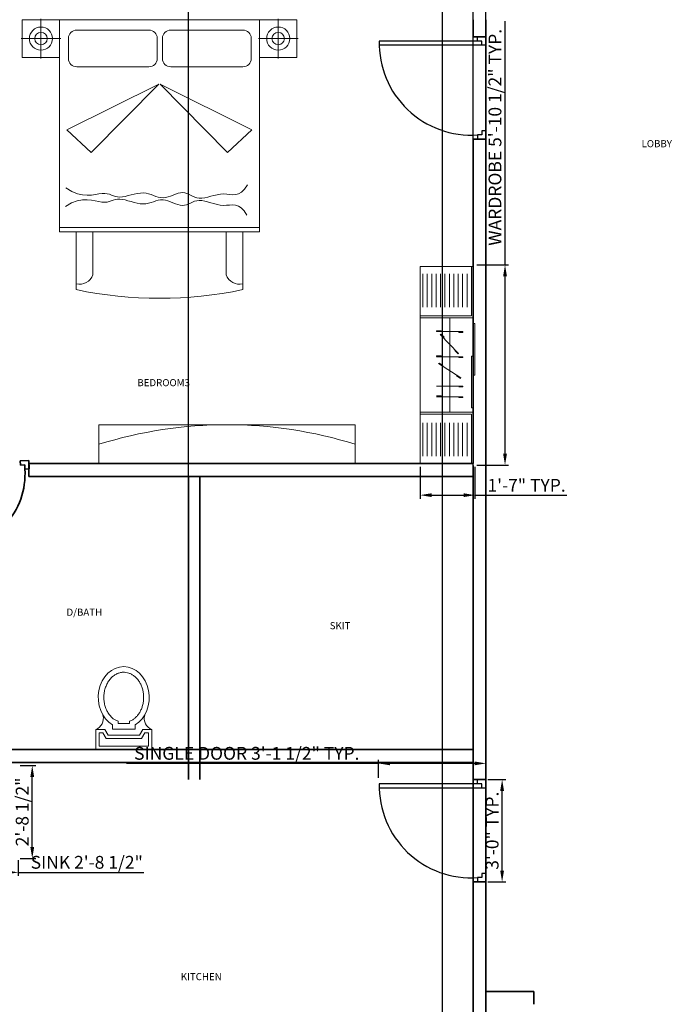
# Model space of a CAD drawing. Units: inches. Extents: x 1239 to 2276906, y 2273 to 321338.
# Tile 16 of 23: x 1392 to 1620, y 3026 to 3372. Entities that reach past the tile are written whole.
import ezdxf

# ---------------------------------------------------------------- set-up
doc = ezdxf.new("R2010")
doc.units = ezdxf.units.IN
for name, color, linetype, lineweight in [('A-ANNO-DIMS', 2, 'Continuous', 18), ('A-AREA-IDEN', 7, 'Continuous', 18), ('A-FLOR-CASE', 8, 'Continuous', 18), ('A-FLOR-FIXT', 9, 'Continuous', 18), ('A-FURN', 8, 'Continuous', 13), ('DOOR', 1, 'Continuous', 25), ('wall', 7, 'Continuous', 35)]:
    doc.layers.add(name, color=color, linetype=linetype, lineweight=lineweight)
doc.styles.get("Standard").update_dxf_attribs({"font": 'arial.ttf'})
doc.dimstyles.new('ISO-25', dxfattribs={"dimtxt": 4.5, "dimasz": 4, "dimexe": 1.25, "dimexo": 0.625, "dimtad": 1, "dimdec": 1, "dimlunit": 3, "dimtxsty": 'Standard', "dimcen": 2.5, "dimadec": 0, "dimazin": 0, "dimtfac": 1, "dimtdec": 1, "dimtmove": 0, "dimatfit": 3, "dimfxl": 1, "dimarcsym": 0})

# ---------------------------------------------------------------- blocks, each defined once
blk = doc.blocks.new('new block')
for p, q in [((1.5, 1.5), (1.5, 30)), ((3, 0), (3, 30)), ((0, 3), (0, 0)), ((1.5, 3), (0, 3)), ((0, 0), (3, 0)), ((1.5, 1.5), (1.5, 3)), ((3, 1.5), (1.5, 1.5)), ((3, 0), (3, 1.5)), ((27, 0), (27, 1.5)), ((27, 1.5), (28.5, 1.5)), ((30, 0), (27, 0)), ((28.5, 1.5), (28.5, 3)), ((28.5, 3), (30, 3)), ((30, 3), (30, 0))]:
    blk.add_line(p, q)
blk.add_arc((2.25, 3.75), 26.26, 358.3634, 91.6366)
blk = doc.blocks.new('2.6door')
at = {"layer": 'wall'}
blk.add_blockref('new block', (0, 0), dxfattribs=at)
blk = doc.blocks.new('A$C4F543DC7')
for p, q in [((0.013, 3.35, -0.169), (3.313, 3.35, -0.169)), ((0.463, 3.35, -0.169), (0.013, 3.35, -0.169)), ((0.013, 2.896, -0.169), (0.013, 3.35, -0.169)), ((0.013, 3.35, -0.169), (0.013, 2.896, -0.169)), ((0.238, 3.123, -0.439), (0.238, 3.361, -0.439)), ((0.463, 3.35, -0.169), (0.463, 0.8, -0.169)), ((2.863, 3.35, -0.169), (0.463, 3.35, -0.169)), ((0.463, 2.896, -0.169), (0.463, 3.35, -0.169)), ((2.863, 0.8, -0.169), (2.863, 3.35, -0.169)), ((2.863, 3.35, -0.169), (3.313, 3.35, -0.169)), ((2.863, 2.896, -0.169), (2.863, 3.35, -0.169)), ((3.089, 3.123, -0.439), (3.089, 3.361, -0.439)), ((3.313, 3.35, -0.169), (3.313, 2.896, -0.169)), ((3.313, 3.35, -0.169), (3.313, 2.896, -0.169)), ((1.535, 3.226, -0.169), (0.668, 3.226, -0.169)), ((2.664, 3.226, -0.169), (1.797, 3.226, -0.169)), ((0.238, 3.123, -0.439), (0, 3.123, -0.439)), ((0.238, 3.123, -0.439), (0.476, 3.123, -0.439)), ((0.238, 3.123, -0.439), (0.238, 2.885, -0.439)), ((0.568, 3.126, -0.169), (0.568, 2.884, -0.169)), ((1.635, 2.884, -0.169), (1.635, 3.126, -0.169)), ((1.697, 3.126, -0.169), (1.697, 2.884, -0.169)), ((2.764, 2.884, -0.169), (2.764, 3.126, -0.169)), ((3.089, 3.123, -0.439), (2.851, 3.123, -0.439)), ((3.089, 3.123, -0.439), (3.089, 2.885, -0.439)), ((3.089, 3.123, -0.439), (3.327, 3.123, -0.439)), ((0.463, 2.896, -0.169), (0.013, 2.896, -0.169)), ((0.013, 2.896, -0.169), (0.463, 2.896, -0.169)), ((0.463, 0.8, -0.169), (0.463, 2.896, -0.169)), ((2.863, 2.896, -0.169), (2.863, 0.8, -0.169)), ((3.313, 2.896, -0.169), (2.863, 2.896, -0.169)), ((3.313, 2.896, -0.169), (2.863, 2.896, -0.169)), ((0.668, 2.784, -0.169), (1.535, 2.784, -0.169)), ((1.797, 2.784, -0.169), (2.664, 2.784, -0.169)), ((1.653, 2.573, -0.169), (0.55, 2.025, -0.169)), ((0.841, 1.752, -0.169), (1.653, 2.573, -0.169)), ((2.481, 1.752, -0.169), (1.669, 2.573, -0.169)), ((1.669, 2.573, -0.169), (2.772, 2.025, -0.169)), ((0.55, 2.025, -0.169), (0.841, 1.752, -0.169)), ((2.772, 2.025, -0.169), (2.481, 1.752, -0.169)), ((0.537, 1.327, -0.169), (0.609, 1.284, -0.169)), ((2.648, 1.277, -0.169), (2.683, 1.312, -0.169)), ((2.683, 1.312, -0.169), (2.718, 1.364, -0.169)), ((0.609, 1.284, -0.169), (0.676, 1.257, -0.169)), ((0.676, 1.257, -0.169), (0.737, 1.243, -0.169)), ((0.736, 1.183, -0.169), (0.793, 1.185, -0.169)), ((0.737, 1.243, -0.169), (0.794, 1.239, -0.169)), ((0.793, 1.185, -0.169), (0.845, 1.18, -0.169)), ((0.794, 1.239, -0.169), (0.846, 1.242, -0.169)), ((0.846, 1.242, -0.169), (0.893, 1.249, -0.169)), ((0.893, 1.249, -0.169), (0.935, 1.256, -0.169)), ((0.935, 1.256, -0.169), (0.972, 1.261, -0.169)), ((0.972, 1.261, -0.169), (1.004, 1.262, -0.169)), ((1.004, 1.262, -0.169), (1.033, 1.258, -0.169)), ((1.033, 1.258, -0.169), (1.06, 1.251, -0.169)), ((1.06, 1.251, -0.169), (1.084, 1.242, -0.169)), ((1.084, 1.242, -0.169), (1.108, 1.234, -0.169)), ((1.107, 1.18, -0.169), (1.132, 1.187, -0.169)), ((1.108, 1.234, -0.169), (1.132, 1.226, -0.169)), ((1.132, 1.226, -0.169), (1.158, 1.22, -0.169)), ((1.132, 1.187, -0.169), (1.157, 1.192, -0.169)), ((1.157, 1.192, -0.169), (1.185, 1.193, -0.169)), ((1.158, 1.22, -0.169), (1.185, 1.218, -0.169)), ((1.185, 1.218, -0.169), (1.216, 1.22, -0.169)), ((1.185, 1.193, -0.169), (1.216, 1.19, -0.169)), ((1.216, 1.22, -0.169), (1.25, 1.226, -0.169)), ((1.216, 1.19, -0.169), (1.249, 1.183, -0.169)), ((1.25, 1.226, -0.169), (1.285, 1.235, -0.169)), ((1.285, 1.235, -0.169), (1.322, 1.244, -0.169)), ((1.322, 1.244, -0.169), (1.359, 1.253, -0.169)), ((1.359, 1.253, -0.169), (1.396, 1.261, -0.169)), ((1.396, 1.261, -0.169), (1.433, 1.266, -0.169)), ((1.433, 1.266, -0.169), (1.468, 1.268, -0.169)), ((1.468, 1.268, -0.169), (1.501, 1.264, -0.169)), ((1.501, 1.264, -0.169), (1.532, 1.257, -0.169)), ((1.532, 1.257, -0.169), (1.562, 1.247, -0.169)), ((1.562, 1.247, -0.169), (1.591, 1.237, -0.169)), ((1.591, 1.237, -0.169), (1.62, 1.226, -0.169)), ((1.62, 1.226, -0.169), (1.648, 1.217, -0.169)), ((1.648, 1.217, -0.169), (1.676, 1.211, -0.169)), ((1.648, 1.18, -0.169), (1.676, 1.185, -0.169)), ((1.676, 1.211, -0.169), (1.705, 1.209, -0.169)), ((1.676, 1.185, -0.169), (1.705, 1.186, -0.169)), ((1.705, 1.209, -0.169), (1.735, 1.212, -0.169)), ((1.705, 1.186, -0.169), (1.734, 1.182, -0.169)), ((1.735, 1.212, -0.169), (1.765, 1.22, -0.169)), ((1.765, 1.22, -0.169), (1.795, 1.23, -0.169)), ((1.795, 1.23, -0.169), (1.826, 1.242, -0.169)), ((1.826, 1.242, -0.169), (1.856, 1.253, -0.169)), ((1.856, 1.253, -0.169), (1.885, 1.263, -0.169)), ((1.885, 1.263, -0.169), (1.913, 1.27, -0.169)), ((1.913, 1.27, -0.169), (1.94, 1.272, -0.169)), ((1.94, 1.272, -0.169), (1.965, 1.269, -0.169)), ((1.965, 1.269, -0.169), (1.989, 1.262, -0.169)), ((1.989, 1.262, -0.169), (2.012, 1.251, -0.169)), ((2.012, 1.251, -0.169), (2.036, 1.239, -0.169)), ((2.036, 1.239, -0.169), (2.06, 1.227, -0.169)), ((2.06, 1.227, -0.169), (2.085, 1.216, -0.169)), ((2.085, 1.216, -0.169), (2.112, 1.208, -0.169)), ((2.112, 1.208, -0.169), (2.141, 1.204, -0.169)), ((2.141, 1.204, -0.169), (2.172, 1.205, -0.169)), ((2.172, 1.205, -0.169), (2.206, 1.21, -0.169)), ((2.206, 1.21, -0.169), (2.242, 1.218, -0.169)), ((2.242, 1.218, -0.169), (2.279, 1.228, -0.169)), ((2.279, 1.228, -0.169), (2.317, 1.238, -0.169)), ((2.317, 1.238, -0.169), (2.356, 1.246, -0.169)), ((2.356, 1.246, -0.169), (2.394, 1.253, -0.169)), ((2.394, 1.253, -0.169), (2.433, 1.255, -0.169)), ((2.433, 1.255, -0.169), (2.47, 1.253, -0.169)), ((2.47, 1.253, -0.169), (2.506, 1.249, -0.169)), ((2.506, 1.249, -0.169), (2.542, 1.246, -0.169)), ((2.542, 1.246, -0.169), (2.578, 1.248, -0.169)), ((2.578, 1.248, -0.169), (2.613, 1.257, -0.169)), ((2.613, 1.257, -0.169), (2.648, 1.277, -0.169)), ((0.533, 1.105, -0.169), (0.607, 1.146, -0.169)), ((0.607, 1.146, -0.169), (0.674, 1.171, -0.169)), ((0.674, 1.171, -0.169), (0.736, 1.183, -0.169)), ((0.845, 1.18, -0.169), (0.891, 1.172, -0.169)), ((0.891, 1.172, -0.169), (0.933, 1.163, -0.169)), ((0.933, 1.163, -0.169), (0.97, 1.156, -0.169)), ((0.97, 1.156, -0.169), (1.003, 1.155, -0.169)), ((1.003, 1.155, -0.169), (1.032, 1.158, -0.169)), ((1.032, 1.158, -0.169), (1.058, 1.164, -0.169)), ((1.058, 1.164, -0.169), (1.083, 1.172, -0.169)), ((1.083, 1.172, -0.169), (1.107, 1.18, -0.169)), ((1.249, 1.183, -0.169), (1.284, 1.173, -0.169)), ((1.284, 1.173, -0.169), (1.321, 1.163, -0.169)), ((1.321, 1.163, -0.169), (1.358, 1.152, -0.169)), ((1.358, 1.152, -0.169), (1.394, 1.143, -0.169)), ((1.394, 1.143, -0.169), (1.431, 1.137, -0.169)), ((1.431, 1.137, -0.169), (1.466, 1.135, -0.169)), ((1.466, 1.135, -0.169), (1.499, 1.137, -0.169)), ((1.499, 1.137, -0.169), (1.531, 1.143, -0.169)), ((1.531, 1.143, -0.169), (1.561, 1.152, -0.169)), ((1.561, 1.152, -0.169), (1.59, 1.162, -0.169)), ((1.59, 1.162, -0.169), (1.619, 1.172, -0.169)), ((1.619, 1.172, -0.169), (1.648, 1.18, -0.169)), ((1.734, 1.182, -0.169), (1.764, 1.173, -0.169)), ((1.764, 1.173, -0.169), (1.794, 1.162, -0.169)), ((1.794, 1.162, -0.169), (1.824, 1.149, -0.169)), ((1.824, 1.149, -0.169), (1.854, 1.137, -0.169)), ((1.854, 1.137, -0.169), (1.883, 1.126, -0.169)), ((1.883, 1.126, -0.169), (1.911, 1.119, -0.169)), ((1.911, 1.119, -0.169), (1.937, 1.115, -0.169)), ((1.937, 1.115, -0.169), (1.963, 1.118, -0.169)), ((1.963, 1.118, -0.169), (1.987, 1.124, -0.169)), ((1.987, 1.124, -0.169), (2.011, 1.134, -0.169)), ((2.011, 1.134, -0.169), (2.034, 1.145, -0.169)), ((2.034, 1.145, -0.169), (2.059, 1.157, -0.169)), ((2.059, 1.157, -0.169), (2.084, 1.167, -0.169)), ((2.084, 1.167, -0.169), (2.111, 1.174, -0.169)), ((2.111, 1.174, -0.169), (2.14, 1.177, -0.169)), ((2.14, 1.177, -0.169), (2.172, 1.175, -0.169)), ((2.172, 1.175, -0.169), (2.206, 1.169, -0.169)), ((2.206, 1.169, -0.169), (2.241, 1.16, -0.169)), ((2.241, 1.16, -0.169), (2.278, 1.149, -0.169)), ((2.278, 1.149, -0.169), (2.316, 1.138, -0.169)), ((2.316, 1.138, -0.169), (2.354, 1.128, -0.169)), ((2.354, 1.128, -0.169), (2.392, 1.121, -0.169)), ((2.392, 1.121, -0.169), (2.43, 1.117, -0.169)), ((2.43, 1.117, -0.169), (2.468, 1.118, -0.169)), ((2.468, 1.118, -0.169), (2.504, 1.121, -0.169)), ((2.504, 1.121, -0.169), (2.54, 1.123, -0.169)), ((2.54, 1.123, -0.169), (2.576, 1.12, -0.169)), ((2.576, 1.12, -0.169), (2.611, 1.109, -0.169)), ((2.611, 1.109, -0.169), (2.645, 1.088, -0.169)), ((2.645, 1.088, -0.169), (2.679, 1.052, -0.169)), ((2.679, 1.052, -0.169), (2.712, 0.999, -0.169)), ((0.463, 0.85, -0.169), (2.863, 0.85, -0.169)), ((0.463, 0.8, -0.169), (2.863, 0.8, -0.169)), ((0.663, 0.8, -0.169), (0.463, 0.8, -0.169)), ((0.663, 0.8, -0.169), (2.663, 0.8, -0.169)), ((0.663, 0.104, -0.169), (0.663, 0.8, -0.169)), ((0.663, 0.104, -0.169), (0.663, 0.8, -0.169)), ((0.863, 0.281, -0.169), (0.863, 0.8, -0.169)), ((2.463, 0.8, -0.169), (2.463, 0.281, -0.169)), ((2.863, 0.8, -0.169), (2.663, 0.8, -0.169)), ((2.663, 0.8, -0.169), (2.663, 0.104, -0.169)), ((2.663, 0.8, -0.169), (2.663, 0.104, -0.169))]:
    blk.add_line(p, q)
for centre, radius in [((0.238, 3.123, -0.439), 0.139), ((0.238, 3.123, -0.439), 0.075), ((3.089, 3.123, -0.439), 0.139), ((3.089, 3.123, -0.439), 0.075)]:
    blk.add_circle(centre, radius)
for centre, radius, start, end in [((0.668, 3.126, -0.169), 0.1, 90, 180), ((1.535, 3.126, -0.169), 0.1, 0, 90), ((1.797, 3.126, -0.169), 0.1, 90, 180), ((2.664, 3.126, -0.169), 0.1, 0, 90), ((0.668, 2.884, -0.169), 0.1, 180, 270), ((1.535, 2.884, -0.169), 0.1, 270, 0), ((1.797, 2.884, -0.169), 0.1, 180, 270), ((2.664, 2.884, -0.169), 0.1, 270, 0), ((0.699, 0.347, -0.169), 0.177, 258.2616, 338.032), ((2.627, 0.347, -0.169), 0.177, 201.968, 281.7384), ((1.663, 4.86, -0.169), 4.86, 258.1252, 281.8748), ((1.663, 4.86, -0.169), 4.86, 258.1252, 281.8748)]:
    blk.add_arc(centre, radius, start, end)
blk = doc.blocks.new('A$C34930FF8')
at = {"ltscale": 0.05}
for p, q in [((0, 2252), (0, 17)), ((600, 2252), (0, 2252)), ((185, 1513), (185, 1521)), ((227, 1479), (233, 1485)), ((238, 1513), (238, 1521)), ((437, 1513), (437, 1504)), ((482, 1513), (482, 1504)), ((264, 1442), (270, 1448)), ((185, 1229), (185, 1238)), ((238, 1229), (238, 1238)), ((398, 1304), (392, 1298)), ((435, 1266), (429, 1260)), ((437, 1228), (437, 1220)), ((482, 1228), (482, 1220)), ((209, 1150), (214, 1157)), ((253, 1122), (258, 1129)), ((415, 1018), (411, 1010)), ((459, 989), (455, 982)), ((482, 895), (482, 886)), ((238, 775), (238, 784)), ((437, 775), (437, 767)), ((482, 775), (482, 767)), ((600, 17), (0, 17))]:
    blk.add_line(p, q, dxfattribs=at)
for p, q in [((580, 1691), (580, 2252)), ((600, 1669), (600, 2269)), ((30, 1791), (30, 2169)), ((80, 1791), (80, 2169)), ((130, 1791), (130, 2169)), ((180, 1791), (180, 2169)), ((230, 1791), (230, 2169)), ((280, 1791), (280, 2169)), ((330, 1791), (330, 2169)), ((380, 1791), (380, 2169)), ((430, 1791), (430, 2169)), ((480, 1791), (480, 2169)), ((530, 1791), (530, 2169)), ((580, 1691), (0, 1691)), ((600, 1669), (0, 1669)), ((335, 1666), (335, 603)), ((600, 1603), (620, 1603)), ((600, 1019), (600, 1603)), ((620, 1603), (620, 1019)), ((238, 1521), (185, 1521)), ((482, 1513), (185, 1513)), ((435, 1266), (227, 1479)), ((270, 1448), (233, 1485)), ((437, 1504), (482, 1504)), ((238, 1238), (185, 1238)), ((482, 1228), (185, 1228)), ((429, 1260), (392, 1298)), ((600, 1233), (580, 1233)), ((580, 1233), (580, 649)), ((600, 649), (600, 1233)), ((459, 989), (209, 1150)), ((258, 1129), (214, 1157)), ((437, 1220), (482, 1220)), ((455, 982), (411, 1010)), ((620, 1019), (600, 1019)), ((482, 895), (185, 895)), ((238, 784), (185, 784)), ((437, 886), (482, 886)), ((482, 775), (185, 775)), ((437, 767), (482, 767)), ((600, 600), (0, 600)), ((580, 578), (0, 578)), ((580, 649), (600, 649)), ((580, 578), (580, 17)), ((600, 600), (600, 0)), ((30, 478), (30, 100)), ((80, 478), (80, 100)), ((130, 478), (130, 100)), ((180, 478), (180, 100)), ((230, 478), (230, 100)), ((280, 478), (280, 100)), ((330, 478), (330, 100)), ((380, 478), (380, 100)), ((430, 478), (430, 100)), ((480, 478), (480, 100)), ((530, 478), (530, 100))]:
    blk.add_line(p, q)
blk = doc.blocks.new('A$C7C8779AE')
for p, q in [((0, 0.7405), (0, 0.5605)), ((0.5, 0.7405), (0, 0.7405)), ((0.47, 0.7105), (0.03, 0.7105)), ((0.03, 0.7105), (0.03, 0.5905)), ((0.47, 0.5905), (0.47, 0.7105)), ((0.5, 0.5605), (0.5, 0.7405)), ((0.093, 0.6405), (0.063, 0.5905)), ((0.093, 0.6405), (0.407, 0.6405)), ((0.437, 0.5905), (0.407, 0.6405)), ((0, 0.5605), (0.08, 0.5605)), ((0.03, 0.5905), (0.063, 0.5905)), ((0.11, 0.6105), (0.08, 0.5605)), ((0.11, 0.6105), (0.39, 0.6105)), ((0.1497, 0.557), (0.1497, 0.5203)), ((0.1497, 0.557), (0.3514, 0.557)), ((0.3514, 0.557), (0.3514, 0.5203)), ((0.42, 0.5605), (0.39, 0.6105)), ((0.42, 0.5605), (0.5, 0.5605)), ((0.437, 0.5905), (0.47, 0.5905)), ((0.1997, 0.507), (0.1997, 0.4879)), ((0.1997, 0.507), (0.3014, 0.507)), ((0.3014, 0.507), (0.3014, 0.4879))]:
    blk.add_line(p, q)
for centre, start, end in [((-0.0386, 0.4613), 344.64203, 68.73386), ((0.5386, 0.4613), 111.26614, 195.35797)]:
    blk.add_arc(centre, 0.1064, start, end)
blk.add_ellipse((0.2506, 0.2744), major_axis=(0, 0.2744), ratio=0.828948, start_param=0.459479, end_param=5.823706)
blk.add_open_spline([(0.1997, 0.4879), (0.1697, 0.474), (0.1642, 0.4702), (0.1512, 0.4602), (0.1438, 0.4535), (0.1298, 0.4388), (0.1233, 0.4306), (0.1111, 0.4131), (0.1055, 0.4037), (0.0956, 0.3838), (0.0912, 0.3733), (0.0838, 0.3516), (0.0808, 0.3403), (0.0762, 0.3172), (0.0746, 0.3055), (0.073, 0.2817), (0.0729, 0.2698), (0.0743, 0.246), (0.0758, 0.2342), (0.0801, 0.2111), (0.0831, 0.1998), (0.0903, 0.1779), (0.0945, 0.1673), (0.1043, 0.1473), (0.1098, 0.1378), (0.1218, 0.12), (0.1283, 0.1118), (0.1421, 0.0968), (0.1494, 0.09), (0.1646, 0.078), (0.1725, 0.0728), (0.1887, 0.064), (0.1969, 0.0603), (0.2137, 0.0547), (0.2222, 0.0527), (0.2392, 0.0502), (0.2478, 0.0498), (0.2664, 0.0505), (0.2764, 0.052), (0.2963, 0.0573), (0.3061, 0.061), (0.3253, 0.0707), (0.3346, 0.0766), (0.3525, 0.0906), (0.3611, 0.0987), (0.3771, 0.1169), (0.3845, 0.127), (0.3978, 0.1488), (0.4037, 0.1605), (0.4137, 0.1853), (0.4178, 0.1983), (0.424, 0.2251), (0.4261, 0.2389), (0.4282, 0.2668), (0.4283, 0.2809), (0.4262, 0.3088), (0.4241, 0.3226), (0.418, 0.3495), (0.414, 0.3625), (0.404, 0.3873), (0.3982, 0.3991), (0.385, 0.421), (0.3776, 0.4311), (0.3617, 0.4494), (0.3531, 0.4575), (0.3382, 0.4693), (0.3321, 0.4736), (0.3014, 0.4879)], degree=3, knots=[0.459479, 0.459479, 0.459479, 0.459479, 0.567422, 0.567422, 0.720865, 0.720865, 0.874307, 0.874307, 1.02775, 1.02775, 1.181192, 1.181192, 1.334635, 1.334635, 1.488077, 1.488077, 1.64152, 1.64152, 1.794963, 1.794963, 1.948405, 1.948405, 2.101848, 2.101848, 2.25529, 2.25529, 2.408733, 2.408733, 2.562175, 2.562175, 2.715618, 2.715618, 2.86906, 2.86906, 3.022503, 3.022503, 3.175946, 3.175946, 3.356457, 3.356457, 3.536968, 3.536968, 3.717479, 3.717479, 3.89799, 3.89799, 4.078501, 4.078501, 4.259012, 4.259012, 4.439523, 4.439523, 4.620035, 4.620035, 4.800546, 4.800546, 4.981057, 4.981057, 5.161568, 5.161568, 5.342079, 5.342079, 5.52259, 5.52259, 5.703101, 5.703101, 5.823706, 5.823706, 5.823706, 5.823706])
blk = doc.blocks.new('DOOR-SINGLE-36')
for p, q in [((33, 1.5), (33, 37.5)), ((34.5, 1.5), (34.5, 37.5)), ((0, 3), (0, 0)), ((1.5, 3), (0, 3)), ((0, 0), (3, 0)), ((1.5, 1.5), (1.5, 3)), ((3, 1.5), (1.5, 1.5)), ((3, 0), (3, 1.5)), ((33, 0), (33, 1.5)), ((33, 1.5), (34.5, 1.5)), ((36, 0), (33, 0)), ((34.5, 1.5), (34.5, 3)), ((34.5, 3), (36, 3)), ((36, 3), (36, 0))]:
    blk.add_line(p, q)
blk.add_arc((33.75, 5.18), 32.32, 88.6705, 183.8756)
blk = doc.blocks.new('*D48')
at = {"layer": 'A-ANNO-DIMS', "color": 0, "lineweight": -2, "transparency": 16777216}
for p, q in [((1518.17, 3111.05), (1429.62, 3111.05)), ((1518.17, 3106.02), (1518.17, 3112.3)), ((1551.88, 3111.05), (1522.17, 3111.05)), ((1555.88, 3106.02), (1555.88, 3112.3))]:
    blk.add_line(p, q, dxfattribs=at)
at = {"layer": 'A-ANNO-DIMS', "color": 0, "transparency": 16777216}
for points in [[(1522.17, 3111.72), (1522.17, 3110.39), (1518.17, 3111.05)], [(1551.88, 3111.72), (1551.88, 3110.39), (1555.88, 3111.05)]]:
    blk.add_solid(points, dxfattribs=at)
at = {"layer": 'Defpoints', "color": 0, "transparency": 16777216}
for p in [(1518.17, 3111.05), (1518.17, 3105.4), (1555.88, 3105.4)]:
    blk.add_point(p, dxfattribs=at)
at = {"layer": 'A-ANNO-DIMS', "color": 0, "transparency": 16777216, "insert": (1471.89, 3114.01), "char_height": 4.5, "attachment_point": 5}
blk.add_mtext('SINGLE DOOR 3\'-1 1/2" TYP.', dxfattribs=at)
blk = doc.blocks.new('*D49')
at = {"layer": 'A-ANNO-DIMS', "color": 0, "lineweight": -2, "transparency": 16777216}
for p, q in [((1556.51, 3105.4), (1562.79, 3105.4)), ((1561.54, 3073.4), (1561.54, 3101.4)), ((1556.51, 3069.4), (1562.79, 3069.4))]:
    blk.add_line(p, q, dxfattribs=at)
at = {"layer": 'A-ANNO-DIMS', "color": 0, "transparency": 16777216}
for points in [[(1560.87, 3101.4), (1562.21, 3101.4), (1561.54, 3105.4)], [(1560.87, 3073.4), (1562.21, 3073.4), (1561.54, 3069.4)]]:
    blk.add_solid(points, dxfattribs=at)
at = {"layer": 'Defpoints', "color": 0, "transparency": 16777216}
for p in [(1555.88, 3105.4), (1561.54, 3105.4), (1555.88, 3069.4)]:
    blk.add_point(p, dxfattribs=at)
at = {"layer": 'A-ANNO-DIMS', "color": 0, "transparency": 16777216, "insert": (1558.62, 3087.4), "char_height": 4.5, "attachment_point": 5, "rotation": 90}
blk.add_mtext('3\'-0" TYP.', dxfattribs=at)
blk = doc.blocks.new('*D66')
at = {"layer": 'A-ANNO-DIMS', "color": 0, "lineweight": -2, "transparency": 16777216}
for p, q in [((1358.99, 3077.03), (1358.99, 3071.51)), ((1391.67, 3077.03), (1391.67, 3071.51)), ((1362.99, 3072.76), (1387.67, 3072.76)), ((1391.67, 3072.76), (1435.76, 3072.76))]:
    blk.add_line(p, q, dxfattribs=at)
at = {"layer": 'A-ANNO-DIMS', "color": 0, "transparency": 16777216}
for points in [[(1362.99, 3073.42), (1362.99, 3072.09), (1358.99, 3072.76)], [(1387.67, 3073.42), (1387.67, 3072.09), (1391.67, 3072.76)]]:
    blk.add_solid(points, dxfattribs=at)
at = {"layer": 'Defpoints', "color": 0, "transparency": 16777216}
for p in [(1358.99, 3077.66), (1391.67, 3077.66), (1391.67, 3072.76)]:
    blk.add_point(p, dxfattribs=at)
at = {"layer": 'A-ANNO-DIMS', "color": 0, "transparency": 16777216, "insert": (1415.71, 3075.71), "char_height": 4.5, "attachment_point": 5}
blk.add_mtext('SINK 2\'-8 1/2"', dxfattribs=at)
blk = doc.blocks.new('*D67')
at = {"layer": 'A-ANNO-DIMS', "color": 0, "lineweight": -2, "transparency": 16777216}
for p, q in [((1392.29, 3110.33), (1397.82, 3110.33)), ((1396.57, 3081.66), (1396.57, 3106.33)), ((1392.29, 3077.66), (1397.82, 3077.66))]:
    blk.add_line(p, q, dxfattribs=at)
at = {"layer": 'A-ANNO-DIMS', "color": 0, "transparency": 16777216}
for points in [[(1395.9, 3106.33), (1397.24, 3106.33), (1396.57, 3110.33)], [(1395.9, 3081.66), (1397.24, 3081.66), (1396.57, 3077.66)]]:
    blk.add_solid(points, dxfattribs=at)
at = {"layer": 'Defpoints', "color": 0, "transparency": 16777216}
for p in [(1391.67, 3110.33), (1396.57, 3110.33), (1391.67, 3077.66)]:
    blk.add_point(p, dxfattribs=at)
at = {"layer": 'A-ANNO-DIMS', "color": 0, "transparency": 16777216, "insert": (1393.62, 3094), "char_height": 4.5, "attachment_point": 5, "rotation": 90}
blk.add_mtext('2\'-8 1/2"', dxfattribs=at)
blk = doc.blocks.new('*D70')
at = {"layer": 'A-ANNO-DIMS', "color": 0, "lineweight": -2, "transparency": 16777216}
for p, q in [((1562.56, 3286.25), (1562.56, 3371.87)), ((1552.63, 3286.25), (1563.81, 3286.25)), ((1562.56, 3219.87), (1562.56, 3282.25)), ((1552.63, 3215.87), (1563.81, 3215.87))]:
    blk.add_line(p, q, dxfattribs=at)
at = {"layer": 'A-ANNO-DIMS', "color": 0, "transparency": 16777216}
for points in [[(1561.89, 3282.25), (1563.23, 3282.25), (1562.56, 3286.25)], [(1561.89, 3219.87), (1563.23, 3219.87), (1562.56, 3215.87)]]:
    blk.add_solid(points, dxfattribs=at)
at = {"layer": 'Defpoints', "color": 0, "transparency": 16777216}
for p in [(1552, 3286.25), (1562.56, 3286.25), (1552, 3215.87)]:
    blk.add_point(p, dxfattribs=at)
at = {"layer": 'A-ANNO-DIMS', "color": 0, "transparency": 16777216, "insert": (1559.61, 3331.06), "char_height": 4.5, "attachment_point": 5, "rotation": 90}
blk.add_mtext('WARDROBE 5\'-10 1/2" TYP.', dxfattribs=at)
blk = doc.blocks.new('*D71')
at = {"layer": 'A-ANNO-DIMS', "color": 0, "lineweight": -2, "transparency": 16777216}
for p, q in [((1532.78, 3215.25), (1532.78, 3204.07)), ((1552, 3215.25), (1552, 3204.07)), ((1536.78, 3205.32), (1548, 3205.32)), ((1552, 3205.32), (1584.26, 3205.32))]:
    blk.add_line(p, q, dxfattribs=at)
at = {"layer": 'A-ANNO-DIMS', "color": 0, "transparency": 16777216}
for points in [[(1536.78, 3205.98), (1536.78, 3204.65), (1532.78, 3205.32)], [(1548, 3205.98), (1548, 3204.65), (1552, 3205.32)]]:
    blk.add_solid(points, dxfattribs=at)
at = {"layer": 'Defpoints', "color": 0, "transparency": 16777216}
for p in [(1532.78, 3215.87), (1552, 3215.87), (1552, 3205.32)]:
    blk.add_point(p, dxfattribs=at)
at = {"layer": 'A-ANNO-DIMS', "color": 0, "transparency": 16777216, "insert": (1570.13, 3208.2), "char_height": 4.5, "attachment_point": 5}
blk.add_mtext('1\'-7" TYP.', dxfattribs=at)
blk = doc.blocks.new('*D89')
at = {"layer": 'A-ANNO-DIMS', "color": 0, "lineweight": -2, "transparency": 16777216}
for p, q in [((1359.38, 3215.77), (1359.38, 2275.7)), ((1551.38, 3215.77), (1551.38, 2275.7)), ((1363.38, 2276.95), (1547.38, 2276.95))]:
    blk.add_line(p, q, dxfattribs=at)
at = {"layer": 'A-ANNO-DIMS', "color": 0, "transparency": 16777216}
for points in [[(1363.38, 2277.61), (1363.38, 2276.28), (1359.38, 2276.95)], [(1547.38, 2277.61), (1547.38, 2276.28), (1551.38, 2276.95)]]:
    blk.add_solid(points, dxfattribs=at)
at = {"layer": 'Defpoints', "color": 0, "transparency": 16777216}
for p in [(1359.38, 3216.4), (1551.38, 3216.4), (1551.38, 2276.95)]:
    blk.add_point(p, dxfattribs=at)
at = {"layer": 'A-ANNO-DIMS', "color": 0, "transparency": 16777216, "insert": (1455.38, 2279.87), "char_height": 4.5, "attachment_point": 5}
blk.add_mtext('16\'-0"', dxfattribs=at)
blk = doc.blocks.new('*D91')
at = {"layer": 'A-ANNO-DIMS', "color": 0, "lineweight": -2, "transparency": 16777216}
for p, q in [((1359.38, 3116.52), (1359.38, 3608.95)), ((1451.38, 3106.02), (1451.38, 3608.95)), ((1363.38, 3607.7), (1447.38, 3607.7))]:
    blk.add_line(p, q, dxfattribs=at)
at = {"layer": 'A-ANNO-DIMS', "color": 0, "transparency": 16777216}
for points in [[(1363.38, 3608.36), (1363.38, 3607.03), (1359.38, 3607.7)], [(1447.38, 3608.36), (1447.38, 3607.03), (1451.38, 3607.7)]]:
    blk.add_solid(points, dxfattribs=at)
at = {"layer": 'Defpoints', "color": 0, "transparency": 16777216}
for p in [(1451.38, 3607.7), (1359.38, 3115.9), (1451.38, 3105.4)]:
    blk.add_point(p, dxfattribs=at)
at = {"layer": 'A-ANNO-DIMS', "color": 0, "transparency": 16777216, "insert": (1405.38, 3610.62), "char_height": 4.5, "attachment_point": 5}
blk.add_mtext('7\'-8"', dxfattribs=at)
blk = doc.blocks.new('*D102')
at = {"layer": 'A-ANNO-DIMS', "color": 0, "lineweight": -2, "transparency": 16777216}
for p, q in [((1317.38, 2608.14), (1317.38, 3608.95)), ((1540.55, 2608.14), (1540.55, 3608.95)), ((1321.38, 3607.7), (1536.55, 3607.7))]:
    blk.add_line(p, q, dxfattribs=at)
at = {"layer": 'A-ANNO-DIMS', "color": 0, "transparency": 16777216}
for points in [[(1321.38, 3608.36), (1321.38, 3607.03), (1317.38, 3607.7)], [(1536.55, 3608.36), (1536.55, 3607.03), (1540.55, 3607.7)]]:
    blk.add_solid(points, dxfattribs=at)
at = {"layer": 'Defpoints', "color": 0, "transparency": 16777216}
for p in [(1540.55, 3607.7), (1317.38, 2607.52), (1540.55, 2607.52)]:
    blk.add_point(p, dxfattribs=at)
at = {"layer": 'A-ANNO-DIMS', "color": 0, "transparency": 16777216, "insert": (1428.97, 3610.62), "char_height": 4.5, "attachment_point": 5}
blk.add_mtext('18\'-7"', dxfattribs=at)
blk = doc.blocks.new('*D111')
at = {"layer": 'A-ANNO-DIMS', "color": 0, "lineweight": -2, "transparency": 16777216}
for p, q in [((1551.38, 2635.52), (1551.38, 3608.95)), ((1555.88, 2631.02), (1555.88, 3608.95)), ((1547.38, 3607.7), (1543.38, 3607.7)), ((1551.38, 3607.7), (1555.88, 3607.7)), ((1559.88, 3607.7), (1587.58, 3607.7))]:
    blk.add_line(p, q, dxfattribs=at)
at = {"layer": 'A-ANNO-DIMS', "color": 0, "transparency": 16777216}
for points in [[(1547.38, 3608.36), (1547.38, 3607.03), (1551.38, 3607.7)], [(1559.88, 3608.36), (1559.88, 3607.03), (1555.88, 3607.7)]]:
    blk.add_solid(points, dxfattribs=at)
at = {"layer": 'Defpoints', "color": 0, "transparency": 16777216}
for p in [(1555.88, 3607.7), (1551.38, 2634.9), (1555.88, 2630.4)]:
    blk.add_point(p, dxfattribs=at)
at = {"layer": 'A-ANNO-DIMS', "color": 0, "transparency": 16777216, "insert": (1575.73, 3610.65), "char_height": 4.5, "attachment_point": 5}
blk.add_mtext('0\'-4 1/2"', dxfattribs=at)
blk = doc.blocks.new('*D112')
at = {"layer": 'A-ANNO-DIMS', "color": 0, "lineweight": -2, "transparency": 16777216}
for p, q in [((1555.88, 3371.77), (1555.88, 2275.7)), ((1661.88, 3371.77), (1661.88, 2275.7)), ((1559.88, 2276.95), (1657.88, 2276.95))]:
    blk.add_line(p, q, dxfattribs=at)
at = {"layer": 'A-ANNO-DIMS', "color": 0, "transparency": 16777216}
for points in [[(1559.88, 2277.61), (1559.88, 2276.28), (1555.88, 2276.95)], [(1657.88, 2277.61), (1657.88, 2276.28), (1661.88, 2276.95)]]:
    blk.add_solid(points, dxfattribs=at)
at = {"layer": 'Defpoints', "color": 0, "transparency": 16777216}
for p in [(1555.88, 3372.4), (1661.88, 3372.4), (1661.88, 2276.95)]:
    blk.add_point(p, dxfattribs=at)
at = {"layer": 'A-ANNO-DIMS', "color": 0, "transparency": 16777216, "insert": (1608.88, 2279.87), "char_height": 4.5, "attachment_point": 5}
blk.add_mtext('8\'-10"', dxfattribs=at)

msp = doc.modelspace()

# ---------------------------------------------------------------- linework, layer by layer
at = {"layer": 'A-FLOR-CASE'}
msp.add_lwpolyline([(1420, 3216.4), (1510, 3216.4), (1510, 3230), (1420, 3230)], close=True, dxfattribs=at)
msp.add_arc((1465, 3079.57), 150.51, 72.6037, 107.3963, dxfattribs=at)
at = {"layer": 'wall'}
for p, q in [((1551.38, 3372.4), (1551.38, 3366.4)), ((1555.88, 3372.4), (1555.88, 3366.4)), ((1551.38, 3366.4), (1555.88, 3366.4)), ((1551.38, 3330.4), (1555.88, 3330.4)), ((1551.38, 3330.4), (1551.38, 3216.4)), ((1555.88, 3330.4), (1555.88, 3205.9)), ((1551.38, 3216.4), (1395.38, 3216.4)), ((1395.38, 3216.4), (1395.38, 3211.9)), ((1551.38, 3211.9), (1395.38, 3211.9)), ((1451.38, 3211.9), (1451.38, 3105.4)), ((1455.38, 3211.9), (1455.38, 3105.4)), ((1551.38, 3211.9), (1551.38, 3205.9)), ((1551.38, 3211.9), (1551.38, 3105.4)), ((1555.88, 3175.9), (1555.88, 3205.9)), ((1555.88, 3175.9), (1555.88, 3105.4)), ((1551.38, 3115.9), (1359.38, 3115.9)), ((1551.38, 3111.4), (1359.38, 3111.4)), ((1551.38, 3105.4), (1555.88, 3105.4)), ((1551.38, 3069.4), (1551.38, 2634.9)), ((1551.38, 3069.4), (1555.88, 3069.4)), ((1555.88, 3069.4), (1555.88, 2855.4)), ((1572.71, 3030.9), (1555.88, 3030.9)), ((1572.71, 3026.4), (1572.71, 3030.9))]:
    msp.add_line(p, q, dxfattribs=at)

# ---------------------------------------------------------------- block references
at = {"layer": 'A-FLOR-CASE', "xscale": 0.031013398049682, "yscale": 0.031013398049682, "zscale": 0.031013398049682}
msp.add_blockref('A$C34930FF8', (1532.78, 3215.87), dxfattribs=at)
at = {"layer": 'A-FLOR-FIXT', "xscale": 39.37007874015748, "yscale": 39.37007874015748, "zscale": 39.37007874015748, "rotation": 180.000000000022}
msp.add_blockref('A$C7C8779AE', (1438.56, 3145.05), dxfattribs=at)
at = {"layer": 'A-FURN', "xscale": 29.2250927527524, "yscale": 29.2250927527524, "zscale": 29.2250927527524}
msp.add_blockref('A$C4F543DC7', (1392.66, 3274.49, 4.93), dxfattribs=at)
at = {"layer": 'DOOR', "rotation": 89.99999999999805}
for p in [(1555.88, 3330.4), (1555.88, 3069.4)]:
    msp.add_blockref('DOOR-SINGLE-36', p, dxfattribs=at)
at = {"layer": 'DOOR', "xscale": -1, "rotation": 182.1398655045003}
msp.add_blockref('2.6door', (1365.38, 3216.4), dxfattribs=at)

# ---------------------------------------------------------------- texts
at = {"layer": 'A-AREA-IDEN', "char_height": 2.5, "attachment_point": 1}
for s, insert in [('LOBBY ', (1610.5, 3330.08)), ('BEDROOM3 ', (1433.46, 3246.1)), ('D/BATH ', (1408.59, 3165.44)), ('SKIT', (1501, 3160.69)), ('KITCHEN ', (1448.71, 3037.37))]:
    msp.add_mtext_dynamic_manual_height_columns(s, width=44.9462, gutter_width=12.5, heights=[0], dxfattribs=dict(at, insert=insert))

# ---------------------------------------------------------------- dimensions: what is measured, and where the dimension line sits
at = {"layer": 'A-ANNO-DIMS'}
for base, p1, p2, picture, middle in [((1555.88, 3607.7), (1551.38, 2634.9), (1555.88, 2630.4), '*D111', (1575.73, 3610.65)), ((1540.55, 3607.7), (1317.38, 2607.52), (1540.55, 2607.52), '*D102', (1428.97, 3610.62)), ((1451.38, 3607.7), (1359.38, 3115.9), (1451.38, 3105.4), '*D91', (1405.38, 3610.62)), ((1661.88, 2276.95), (1555.88, 3372.4), (1661.88, 3372.4), '*D112', (1608.88, 2279.87)), ((1551.38, 2276.95), (1359.38, 3216.4), (1551.38, 3216.4), '*D89', (1455.38, 2279.87))]:
    dim = msp.add_linear_dim(base=base, p1=p1, p2=p2, dimstyle='ISO-25', override={"dimdec": 1, "dimlfac": 1, "dimrnd": 0, "dimzin": 1, "dimdsep": 46, "dimlunit": 4, "dimfrac": 2}, dxfattribs=at)
    dim.commit()
    dim.dimension.update_dxf_attribs({"geometry": picture, "text_midpoint": middle})
for base, p1, p2, angle, text, picture, middle in [((1562.56, 3286.25), (1552, 3215.87), (1552, 3286.25), 90, 'WARDROBE <> TYP.', '*D70', (1559.61, 3331.06)), ((1518.17, 3111.05), (1555.88, 3105.4), (1518.17, 3105.4), 180, 'SINGLE DOOR <> TYP.', '*D48', (1471.89, 3114.01)), ((1561.54, 3105.4), (1555.88, 3069.4), (1555.88, 3105.4), 90, '<> TYP.', '*D49', (1558.62, 3087.4))]:
    dim = msp.add_linear_dim(base=base, p1=p1, p2=p2, angle=angle, text=text, dimstyle='ISO-25', override={"dimdec": 1, "dimlfac": 1, "dimrnd": 0, "dimzin": 1, "dimdsep": 46, "dimlunit": 4, "dimfrac": 2}, dxfattribs=at)
    dim.commit()
    dim.dimension.update_dxf_attribs({"geometry": picture, "text_midpoint": middle})
for base, p1, p2, text, picture, middle in [((1552, 3205.32), (1532.78, 3215.87), (1552, 3215.87), '<> TYP.', '*D71', (1570.13, 3208.2)), ((1391.67, 3072.76), (1358.99, 3077.66), (1391.67, 3077.66), 'SINK <>', '*D66', (1415.71, 3075.71))]:
    dim = msp.add_linear_dim(base=base, p1=p1, p2=p2, text=text, dimstyle='ISO-25', override={"dimdec": 1, "dimlfac": 1, "dimrnd": 0, "dimzin": 1, "dimdsep": 46, "dimlunit": 4, "dimfrac": 2}, dxfattribs=at)
    dim.commit()
    dim.dimension.update_dxf_attribs({"geometry": picture, "text_midpoint": middle})
dim = msp.add_linear_dim(base=(1396.57, 3110.33), p1=(1391.67, 3077.66), p2=(1391.67, 3110.33), angle=90, dimstyle='ISO-25', override={"dimdec": 1, "dimlfac": 1, "dimrnd": 0, "dimzin": 1, "dimdsep": 46, "dimlunit": 4, "dimfrac": 2}, dxfattribs=at)
dim.commit()
dim.dimension.update_dxf_attribs({"geometry": '*D67', "text_midpoint": (1393.62, 3094)})

doc.saveas('drawing.dxf')
